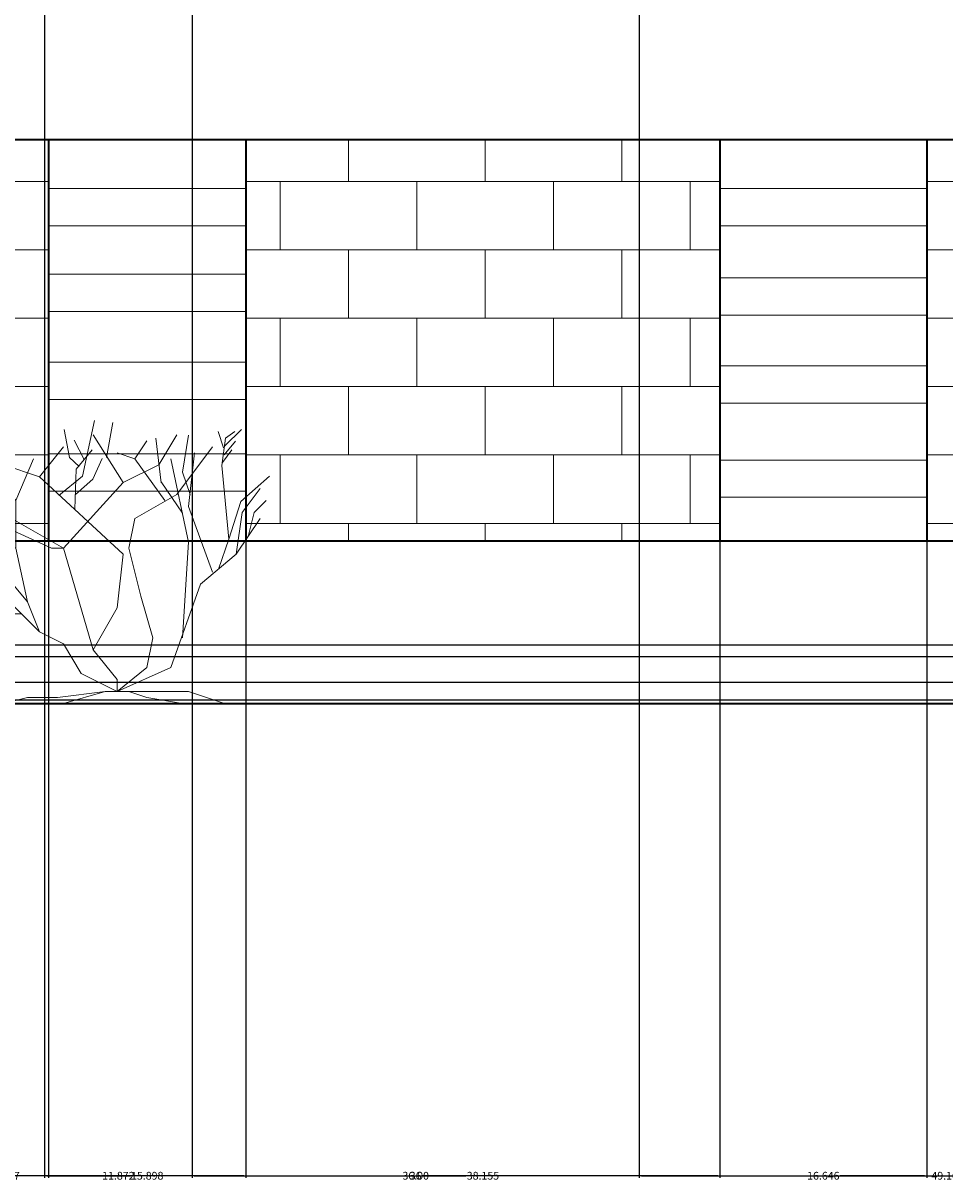
# Model space of a CAD drawing. Units: inches. Extents: x -13 to 809, y 112 to 656.
# Tile 7 of 55: x 111 to 186, y 112 to 205. Entities that reach past the tile are written whole.
import ezdxf

# ---------------------------------------------------------------- set-up
doc = ezdxf.new("R2010")
doc.units = ezdxf.units.IN
doc.header["$MEASUREMENT"] = 0
for name, color, linetype, lineweight in [('A-ANNO-DIMS', 2, 'Continuous', 18), ('A-ELEV', 7, 'Continuous', 35), ('A-ELEV-PATT', 8, 'Continuous', 13), ('L-PLNT', 3, 'Continuous', 18)]:
    doc.layers.add(name, color=color, linetype=linetype, lineweight=lineweight)
doc.styles.get("Standard").update_dxf_attribs({"font": 'arial.ttf'})
doc.dimstyles.get("Standard").update_dxf_attribs({"dimtxt": 0.625, "dimasz": 0.18, "dimexe": 0.18, "dimexo": 0.0625, "dimgap": 0.09, "dimtad": 0, "dimtih": 1, "dimtoh": 1, "dimdec": 4, "dimzin": 0, "dimdsep": 46, "dimlunit": 4, "dimtxsty": 'Standard', "dimcen": 0.09, "dimadec": 0, "dimazin": 0, "dimtfac": 1, "dimtdec": 4, "dimtofl": 0, "dimtmove": 0, "dimatfit": 3, "dimfxl": 1, "dimtolj": 1, "dimtzin": 0, "dimarcsym": 0})

# ---------------------------------------------------------------- blocks, each defined once
blk = doc.blocks.new('Shrub - elevation')
for p, q in [((-11.433, 18.289), (-10.457, 22.749)), ((-9.48, 19.775), (-8.992, 22.592)), ((-12.471, 19.775), (-12.898, 22.044)), ((-8.16, 17.76), (-10.56, 21.6)), ((-5.28, 19.2), (-3.84, 21.6)), ((-3.377, 18.602), (-2.888, 21.575)), ((-0.508, 21.888), (-0.081, 20.558)), ((0.041, 20.714), (1.384, 22.044)), ((0.102, 21.34), (0.835, 21.888)), ((-14.88, 18.24), (-12.96, 20.64)), ((-11.28, 19.619), (-12.104, 21.184)), ((-7.2, 19.68), (-6.24, 21.12)), ((-5.086, 17.741), (-5.513, 21.34)), ((-3.84, 16.8), (-0.96, 20.64)), ((-0.203, 19.149), (0.102, 21.34)), ((-0.02, 20.01), (0.896, 21.105)), ((-16.8, 16.32), (-15.36, 19.68)), ((-11.677, 19.071), (-12.471, 19.775)), ((-11.921, 18.836), (-10.64, 20.401)), ((-10.579, 18.054), (-9.846, 19.697)), ((-7.2, 19.68), (-8.64, 20.16)), ((-4.8, 16.32), (-7.2, 19.68)), ((-2.88, 12.96), (-4.32, 19.68)), ((-2.88, 15.84), (-2.4, 20.16)), ((-0.142, 19.384), (0.59, 20.401)), ((-16.8, 16.32), (-18.72, 18.72)), ((-14.88, 18.24), (-17.76, 19.2)), ((-12.043, 15.628), (-11.921, 18.836)), ((-8.16, 17.76), (-5.28, 19.2)), ((0.346, 13.203), (-0.203, 19.149)), ((-8.16, 12), (-14.88, 18.24)), ((-13.325, 16.724), (-11.433, 18.289)), ((-12.96, 12.48), (-8.16, 17.76)), ((-11.982, 16.802), (-10.579, 18.054)), ((-3.377, 15.315), (-5.086, 17.819)), ((-2.766, 16.802), (-3.377, 18.602)), ((1.323, 16.254), (3.642, 18.289)), ((-7.2, 14.88), (-3.84, 16.8)), ((1.44, 15.36), (2.88, 17.28)), ((-18.24, 11.04), (-21.755, 16.655)), ((-12.96, 12.48), (-19.68, 16.32)), ((-16.8, 12.48), (-16.8, 16.32)), ((-0.96, 10.56), (-2.88, 15.84)), ((0.346, 13.203), (1.323, 16.254)), ((2.4, 15.36), (3.36, 16.32)), ((0.96, 12), (1.44, 15.36)), ((1.92, 13.44), (2.4, 15.36)), ((-13.92, 12.48), (-19.2, 14.88)), ((-7.68, 12.48), (-7.2, 14.88)), ((0.96, 12), (2.88, 14.88)), ((-0.48, 10.8), (0.346, 13.203)), ((-16.8, 12.48), (-17.76, 12.96)), ((-15.84, 8.16), (-16.8, 12.48)), ((-12.96, 12.48), (-13.92, 12.48)), ((-10.56, 4.32), (-12.96, 12.48)), ((-6.72, 8.64), (-7.68, 12.48)), ((-3.36, 5.28), (-2.88, 12.96)), ((-17.76, 8.64), (-23.663, 11.961)), ((-18.24, 11.04), (-20.16, 11.52)), ((-8.64, 7.68), (-8.16, 12)), ((-1.92, 9.6), (0.96, 12)), ((-15.84, 8.16), (-18.24, 11.04)), ((-4.32, 2.88), (-1.92, 9.6)), ((-17.76, 8.64), (-23.128, 9.222)), ((-14.88, 5.76), (-17.76, 8.64)), ((-5.76, 5.28), (-6.72, 8.64)), ((-14.88, 5.76), (-15.84, 8.16)), ((-10.56, 4.32), (-8.64, 7.68)), ((-16.32, 7.2), (-18.24, 7.2)), ((-12.96, 4.8), (-14.88, 5.76)), ((-11.52, 2.4), (-12.96, 4.8)), ((-6.24, 2.88), (-5.76, 5.28)), ((-8.64, 1.92), (-10.56, 4.32)), ((-8.64, 0.96), (-4.32, 2.88)), ((-8.64, 0.96), (-6.24, 2.88)), ((-8.64, 0.96), (-11.52, 2.4)), ((-8.64, 0.96), (-8.64, 1.92)), ((-9.6, 0.96), (-13.44, 0.48)), ((-9.6, 0.96), (-12.96, 0)), ((-9.6, 0.96), (-7.68, 0.96)), ((-8.64, 0.96), (-2.88, 0.96)), ((-7.68, 0.96), (-6.24, 0.48)), ((-2.88, 0.96), (0, 0)), ((-15.84, 0.48), (-17.76, 0)), ((-13.44, 0.48), (-15.84, 0.48)), ((-6.24, 0.48), (-3.36, 0))]:
    blk.add_line(p, q)
blk = doc.blocks.new('*D12')
at = {"layer": 'A-ANNO-DIMS', "color": 0, "lineweight": -2, "transparency": 16777216}
for p, q in [((95.047, 306.457), (95.047, 112.34)), ((124.918, 210.457), (124.918, 112.34)), ((95.227, 112.52), (108.833, 112.52)), ((124.738, 112.52), (111.133, 112.52))]:
    blk.add_line(p, q, dxfattribs=at)
at = {"layer": 'A-ANNO-DIMS', "color": 0, "transparency": 16777216}
for points in [[(95.227, 112.55), (95.227, 112.49), (95.047, 112.52)], [(124.738, 112.55), (124.738, 112.49), (124.918, 112.52)]]:
    blk.add_solid(points, dxfattribs=at)
at = {"layer": 'Defpoints', "color": 0, "transparency": 16777216}
for p in [(95.047, 306.52), (124.918, 210.52), (124.918, 112.52)]:
    blk.add_point(p, dxfattribs=at)
at = {"layer": 'A-ANNO-DIMS', "color": 0, "transparency": 16777216, "insert": (109.983, 112.52), "char_height": 0.625, "attachment_point": 5}
blk.add_mtext('\\A1;29.87', dxfattribs=at)
blk = doc.blocks.new('*D13')
at = {"layer": 'A-ANNO-DIMS', "color": 0, "lineweight": -2, "transparency": 16777216}
for p, q in [((124.918, 210.457), (124.918, 112.34)), ((160.918, 210.457), (160.918, 112.34)), ((125.098, 112.52), (142.381, 112.52)), ((160.738, 112.52), (143.456, 112.52))]:
    blk.add_line(p, q, dxfattribs=at)
at = {"layer": 'A-ANNO-DIMS', "color": 0, "transparency": 16777216}
for points in [[(125.098, 112.55), (125.098, 112.49), (124.918, 112.52)], [(160.738, 112.55), (160.738, 112.49), (160.918, 112.52)]]:
    blk.add_solid(points, dxfattribs=at)
at = {"layer": 'Defpoints', "color": 0, "transparency": 16777216}
for p in [(124.918, 210.52), (160.918, 210.52), (160.918, 112.52)]:
    blk.add_point(p, dxfattribs=at)
at = {"layer": 'A-ANNO-DIMS', "color": 0, "transparency": 16777216, "insert": (142.918, 112.52), "char_height": 0.625, "attachment_point": 5}
blk.add_mtext('\\A1;36', dxfattribs=at)
blk = doc.blocks.new('*D14')
at = {"layer": 'A-ANNO-DIMS', "color": 0, "lineweight": -2, "transparency": 16777216}
for p, q in [((210.079, 223.038), (210.079, 112.34)), ((160.918, 210.457), (160.918, 112.34)), ((161.098, 112.52), (184.342, 112.52)), ((209.899, 112.52), (186.656, 112.52))]:
    blk.add_line(p, q, dxfattribs=at)
at = {"layer": 'A-ANNO-DIMS', "color": 0, "transparency": 16777216}
for points in [[(161.098, 112.55), (161.098, 112.49), (160.918, 112.52)], [(209.899, 112.55), (209.899, 112.49), (210.079, 112.52)]]:
    blk.add_solid(points, dxfattribs=at)
at = {"layer": 'Defpoints', "color": 0, "transparency": 16777216}
for p in [(210.079, 223.1), (160.918, 210.52), (210.079, 112.52)]:
    blk.add_point(p, dxfattribs=at)
at = {"layer": 'A-ANNO-DIMS', "color": 0, "transparency": 16777216, "insert": (185.499, 112.52), "char_height": 0.625, "attachment_point": 5}
blk.add_mtext('\\A1;49.16', dxfattribs=at)
blk = doc.blocks.new('*D85')
at = {"layer": 'A-ANNO-DIMS', "color": 0, "lineweight": -2, "transparency": 16777216}
for p, q in [((76.473, 195.828), (76.473, 112.34)), ((113.357, 195.828), (113.357, 112.34)), ((76.653, 112.52), (93.529, 112.52)), ((113.177, 112.52), (96.301, 112.52))]:
    blk.add_line(p, q, dxfattribs=at)
at = {"layer": 'A-ANNO-DIMS', "color": 0, "transparency": 16777216}
for points in [[(76.653, 112.55), (76.653, 112.49), (76.473, 112.52)], [(113.177, 112.55), (113.177, 112.49), (113.357, 112.52)]]:
    blk.add_solid(points, dxfattribs=at)
at = {"layer": 'Defpoints', "color": 0, "transparency": 16777216}
for p in [(76.473, 195.891), (113.357, 195.891), (113.357, 112.52)]:
    blk.add_point(p, dxfattribs=at)
at = {"layer": 'A-ANNO-DIMS', "color": 0, "transparency": 16777216, "insert": (94.915, 112.52), "char_height": 0.625, "attachment_point": 5}
blk.add_mtext('\\A1;36.884', dxfattribs=at)
blk = doc.blocks.new('*D86')
at = {"layer": 'A-ANNO-DIMS', "color": 0, "lineweight": -2, "transparency": 16777216}
for p, q in [((113.357, 195.828), (113.357, 112.34)), ((129.255, 195.828), (129.255, 112.34)), ((113.537, 112.52), (119.948, 112.52)), ((129.075, 112.52), (122.665, 112.52))]:
    blk.add_line(p, q, dxfattribs=at)
at = {"layer": 'A-ANNO-DIMS', "color": 0, "transparency": 16777216}
for points in [[(113.537, 112.55), (113.537, 112.49), (113.357, 112.52)], [(129.075, 112.55), (129.075, 112.49), (129.255, 112.52)]]:
    blk.add_solid(points, dxfattribs=at)
at = {"layer": 'Defpoints', "color": 0, "transparency": 16777216}
for p in [(113.357, 195.891), (129.255, 195.891), (129.255, 112.52)]:
    blk.add_point(p, dxfattribs=at)
at = {"layer": 'A-ANNO-DIMS', "color": 0, "transparency": 16777216, "insert": (121.306, 112.52), "char_height": 0.625, "attachment_point": 5}
blk.add_mtext('\\A1;15.898', dxfattribs=at)
blk = doc.blocks.new('*D87')
at = {"layer": 'A-ANNO-DIMS', "color": 0, "lineweight": -2, "transparency": 16777216}
for p, q in [((129.255, 195.828), (129.255, 112.34)), ((167.41, 195.828), (167.41, 112.34)), ((129.435, 112.52), (146.943, 112.52)), ((167.23, 112.52), (149.722, 112.52))]:
    blk.add_line(p, q, dxfattribs=at)
at = {"layer": 'A-ANNO-DIMS', "color": 0, "transparency": 16777216}
for points in [[(129.435, 112.55), (129.435, 112.49), (129.255, 112.52)], [(167.23, 112.55), (167.23, 112.49), (167.41, 112.52)]]:
    blk.add_solid(points, dxfattribs=at)
at = {"layer": 'Defpoints', "color": 0, "transparency": 16777216}
for p in [(129.255, 195.891), (167.41, 195.891), (167.41, 112.52)]:
    blk.add_point(p, dxfattribs=at)
at = {"layer": 'A-ANNO-DIMS', "color": 0, "transparency": 16777216, "insert": (148.332, 112.52), "char_height": 0.625, "attachment_point": 5}
blk.add_mtext('\\A1;38.155', dxfattribs=at)
blk = doc.blocks.new('*D88')
at = {"layer": 'A-ANNO-DIMS', "color": 0, "lineweight": -2, "transparency": 16777216}
for p, q in [((167.41, 195.828), (167.41, 112.34)), ((184.056, 195.828), (184.056, 112.34)), ((167.59, 112.52), (174.375, 112.52)), ((183.876, 112.52), (177.09, 112.52))]:
    blk.add_line(p, q, dxfattribs=at)
at = {"layer": 'A-ANNO-DIMS', "color": 0, "transparency": 16777216}
for points in [[(167.59, 112.55), (167.59, 112.49), (167.41, 112.52)], [(183.876, 112.55), (183.876, 112.49), (184.056, 112.52)]]:
    blk.add_solid(points, dxfattribs=at)
at = {"layer": 'Defpoints', "color": 0, "transparency": 16777216}
for p in [(167.41, 195.891), (184.056, 195.891), (184.056, 112.52)]:
    blk.add_point(p, dxfattribs=at)
at = {"layer": 'A-ANNO-DIMS', "color": 0, "transparency": 16777216, "insert": (175.733, 112.52), "char_height": 0.625, "attachment_point": 5}
blk.add_mtext('\\A1;16.646', dxfattribs=at)
blk = doc.blocks.new('*D89')
at = {"layer": 'A-ANNO-DIMS', "color": 0, "lineweight": -2, "transparency": 16777216}
for p, q in [((184.056, 195.828), (184.056, 112.34)), ((229.674, 195.828), (229.674, 112.34)), ((184.236, 112.52), (205.711, 112.52)), ((229.494, 112.52), (208.019, 112.52))]:
    blk.add_line(p, q, dxfattribs=at)
at = {"layer": 'A-ANNO-DIMS', "color": 0, "transparency": 16777216}
for points in [[(184.236, 112.55), (184.236, 112.49), (184.056, 112.52)], [(229.494, 112.55), (229.494, 112.49), (229.674, 112.52)]]:
    blk.add_solid(points, dxfattribs=at)
at = {"layer": 'Defpoints', "color": 0, "transparency": 16777216}
for p in [(184.056, 195.891), (229.674, 195.891), (229.674, 112.52)]:
    blk.add_point(p, dxfattribs=at)
at = {"layer": 'A-ANNO-DIMS', "color": 0, "transparency": 16777216, "insert": (206.865, 112.52), "char_height": 0.625, "attachment_point": 5}
blk.add_mtext('\\A1;45.62', dxfattribs=at)
blk = doc.blocks.new('*D107')
at = {"layer": 'A-ANNO-DIMS', "color": 0, "lineweight": -2, "transparency": 16777216}
for p, q in [((113.047, 324.457), (113.047, 112.34)), ((95.047, 306.457), (95.047, 112.34)), ((95.227, 112.52), (102.933, 112.52)), ((112.867, 112.52), (105.161, 112.52))]:
    blk.add_line(p, q, dxfattribs=at)
at = {"layer": 'A-ANNO-DIMS', "color": 0, "transparency": 16777216}
for points in [[(95.227, 112.55), (95.227, 112.49), (95.047, 112.52)], [(112.867, 112.55), (112.867, 112.49), (113.047, 112.52)]]:
    blk.add_solid(points, dxfattribs=at)
at = {"layer": 'Defpoints', "color": 0, "transparency": 16777216}
for p in [(113.047, 324.52), (95.047, 306.52), (113.047, 112.52)]:
    blk.add_point(p, dxfattribs=at)
at = {"layer": 'A-ANNO-DIMS', "color": 0, "transparency": 16777216, "insert": (104.047, 112.52), "char_height": 0.625, "attachment_point": 5}
blk.add_mtext('\\A1;18.00', dxfattribs=at)
blk = doc.blocks.new('*D109')
at = {"layer": 'A-ANNO-DIMS', "color": 0, "lineweight": -2, "transparency": 16777216}
for p, q in [((113.047, 324.457), (113.047, 112.34)), ((124.918, 324.457), (124.918, 112.34)), ((113.227, 112.52), (117.628, 112.52)), ((124.738, 112.52), (120.337, 112.52))]:
    blk.add_line(p, q, dxfattribs=at)
at = {"layer": 'A-ANNO-DIMS', "color": 0, "transparency": 16777216}
for points in [[(113.227, 112.55), (113.227, 112.49), (113.047, 112.52)], [(124.738, 112.55), (124.738, 112.49), (124.918, 112.52)]]:
    blk.add_solid(points, dxfattribs=at)
at = {"layer": 'Defpoints', "color": 0, "transparency": 16777216}
for p in [(113.047, 324.52), (124.918, 324.52), (124.918, 112.52)]:
    blk.add_point(p, dxfattribs=at)
at = {"layer": 'A-ANNO-DIMS', "color": 0, "transparency": 16777216, "insert": (118.983, 112.52), "char_height": 0.625, "attachment_point": 5}
blk.add_mtext('\\A1;11.872', dxfattribs=at)
blk = doc.blocks.new('*D110')
at = {"layer": 'A-ANNO-DIMS', "color": 0, "lineweight": -2, "transparency": 16777216}
for p, q in [((124.918, 324.457), (124.918, 112.34)), ((160.918, 324.457), (160.918, 112.34)), ((125.098, 112.52), (141.775, 112.52)), ((160.738, 112.52), (144.062, 112.52))]:
    blk.add_line(p, q, dxfattribs=at)
at = {"layer": 'A-ANNO-DIMS', "color": 0, "transparency": 16777216}
for points in [[(125.098, 112.55), (125.098, 112.49), (124.918, 112.52)], [(160.738, 112.55), (160.738, 112.49), (160.918, 112.52)]]:
    blk.add_solid(points, dxfattribs=at)
at = {"layer": 'Defpoints', "color": 0, "transparency": 16777216}
for p in [(124.918, 324.52), (160.918, 324.52), (160.918, 112.52)]:
    blk.add_point(p, dxfattribs=at)
at = {"layer": 'A-ANNO-DIMS', "color": 0, "transparency": 16777216, "insert": (142.918, 112.52), "char_height": 0.625, "attachment_point": 5}
blk.add_mtext('\\A1;36.00', dxfattribs=at)
blk = doc.blocks.new('*D111')
at = {"layer": 'A-ANNO-DIMS', "color": 0, "lineweight": -2, "transparency": 16777216}
for p, q in [((210.079, 361.229), (210.079, 112.34)), ((160.918, 324.457), (160.918, 112.34)), ((161.098, 112.52), (184.342, 112.52)), ((209.899, 112.52), (186.656, 112.52))]:
    blk.add_line(p, q, dxfattribs=at)
at = {"layer": 'A-ANNO-DIMS', "color": 0, "transparency": 16777216}
for points in [[(161.098, 112.55), (161.098, 112.49), (160.918, 112.52)], [(209.899, 112.55), (209.899, 112.49), (210.079, 112.52)]]:
    blk.add_solid(points, dxfattribs=at)
at = {"layer": 'Defpoints', "color": 0, "transparency": 16777216}
for p in [(210.079, 361.292), (160.918, 324.52), (210.079, 112.52)]:
    blk.add_point(p, dxfattribs=at)
at = {"layer": 'A-ANNO-DIMS', "color": 0, "transparency": 16777216, "insert": (185.499, 112.52), "char_height": 0.625, "attachment_point": 5}
blk.add_mtext('\\A1;49.16', dxfattribs=at)
blk = doc.blocks.new('*D115')
at = {"layer": 'A-ANNO-DIMS', "color": 0, "lineweight": -2, "transparency": 16777216}
for p, q in [((311.4, 210.785), (-12.099, 210.785)), ((-11.919, 210.605), (-11.919, 181.062)), ((-11.919, 150.7), (-11.919, 180.243)), ((311.637, 150.52), (-12.099, 150.52))]:
    blk.add_line(p, q, dxfattribs=at)
at = {"layer": 'A-ANNO-DIMS', "color": 0, "transparency": 16777216}
for points in [[(-11.949, 210.605), (-11.889, 210.605), (-11.919, 210.785)], [(-11.949, 150.7), (-11.889, 150.7), (-11.919, 150.52)]]:
    blk.add_solid(points, dxfattribs=at)
at = {"layer": 'Defpoints', "color": 0, "transparency": 16777216}
for p in [(-11.919, 210.785), (311.463, 210.785), (311.699, 150.52)]:
    blk.add_point(p, dxfattribs=at)
at = {"layer": 'A-ANNO-DIMS', "color": 0, "transparency": 16777216, "insert": (-11.919, 180.652), "char_height": 0.625, "attachment_point": 5}
blk.add_mtext('\\A1;60.27', dxfattribs=at)
blk = doc.blocks.new('*D117')
at = {"layer": 'A-ANNO-DIMS', "color": 0, "lineweight": -2, "transparency": 16777216}
for p, q in [((260.642, 154.272), (-12.099, 154.272)), ((-11.919, 154.092), (-11.919, 152.938)), ((-11.919, 150.965), (-11.919, 152.119)), ((258.04, 150.785), (-12.099, 150.785))]:
    blk.add_line(p, q, dxfattribs=at)
at = {"layer": 'A-ANNO-DIMS', "color": 0, "transparency": 16777216}
for points in [[(-11.949, 154.092), (-11.889, 154.092), (-11.919, 154.272)], [(-11.949, 150.965), (-11.889, 150.965), (-11.919, 150.785)]]:
    blk.add_solid(points, dxfattribs=at)
at = {"layer": 'Defpoints', "color": 0, "transparency": 16777216}
for p in [(260.705, 154.272), (-11.919, 150.785), (258.102, 150.785)]:
    blk.add_point(p, dxfattribs=at)
at = {"layer": 'A-ANNO-DIMS', "color": 0, "transparency": 16777216, "insert": (-11.919, 152.529), "char_height": 0.625, "attachment_point": 5}
blk.add_mtext('\\A1;3.487', dxfattribs=at)
blk = doc.blocks.new('*D131')
at = {"layer": 'A-ANNO-DIMS', "color": 0, "lineweight": -2, "transparency": 16777216}
for p, q in [((368.876, 155.214), (-12.099, 155.214)), ((-11.919, 155.034), (-11.919, 154.123)), ((-11.919, 152.394), (-11.919, 153.305)), ((365.876, 152.214), (-12.099, 152.214))]:
    blk.add_line(p, q, dxfattribs=at)
at = {"layer": 'A-ANNO-DIMS', "color": 0, "transparency": 16777216}
for points in [[(-11.949, 155.034), (-11.889, 155.034), (-11.919, 155.214)], [(-11.949, 152.394), (-11.889, 152.394), (-11.919, 152.214)]]:
    blk.add_solid(points, dxfattribs=at)
at = {"layer": 'Defpoints', "color": 0, "transparency": 16777216}
for p in [(368.938, 155.214), (-11.919, 152.214), (365.938, 152.214)]:
    blk.add_point(p, dxfattribs=at)
at = {"layer": 'A-ANNO-DIMS', "color": 0, "transparency": 16777216, "insert": (-11.919, 153.714), "char_height": 0.625, "attachment_point": 5}
blk.add_mtext('\\A1;3.00', dxfattribs=at)

msp = doc.modelspace()

# ---------------------------------------------------------------- hatches: boundary and pattern name
at = {"layer": 'A-ELEV-PATT'}
h = msp.add_hatch(dxfattribs=at)
h.set_pattern_fill('BRICK', color=256, scale=22)
h.paths.add_polyline_path([(113.3574, 195.8907), (76.4733, 195.8907), (76.4733, 163.5637), (113.3574, 163.5637)])
h.paths.add_polyline_path([(167.4098, 195.8907), (129.2551, 195.8907), (129.2551, 163.5637), (167.4098, 163.5637)])
h.paths.add_polyline_path([(229.6736, 195.8907), (184.0557, 195.8907), (184.0557, 163.5637), (229.6736, 163.5637)])

# ---------------------------------------------------------------- linework, layer by layer
at = {"layer": 'A-ELEV'}
for p, q in [((113.3574, 195.8907), (113.3574, 163.5637)), ((129.2551, 195.8907), (129.2551, 163.5637)), ((167.4098, 195.8907), (167.4098, 163.5637)), ((184.0557, 195.8907), (184.0557, 163.5637)), ((109.5888, 150.5199), (649.5888, 150.5199))]:
    msp.add_line(p, q, dxfattribs=at)
msp.add_lwpolyline([(76.4733, 195.8907), (229.6736, 195.8907), (229.6736, 163.5637), (76.4733, 163.5637)], close=True, dxfattribs=at)
at = {"layer": 'A-ELEV-PATT'}
for p, q in [((113.3574, 191.9338), (129.2551, 191.9338)), ((167.4098, 191.9338), (184.0557, 191.9338)), ((113.3574, 188.9338), (129.2551, 188.9338)), ((167.4098, 188.9338), (184.0557, 188.9338)), ((113.3574, 185.0499), (129.2551, 185.0499)), ((167.4098, 184.7549), (184.0557, 184.7549)), ((113.3574, 182.0499), (129.2551, 182.0499)), ((167.4098, 181.7549), (184.0557, 181.7549)), ((113.3574, 177.9693), (129.2551, 177.9693)), ((167.4098, 177.6743), (184.0557, 177.6743)), ((113.3574, 174.9693), (129.2551, 174.9693)), ((167.4098, 174.6743), (184.0557, 174.6743)), ((113.3574, 170.5937), (129.2551, 170.5937)), ((167.4098, 170.102), (184.0557, 170.102)), ((113.3574, 167.5937), (129.2551, 167.5937)), ((167.4098, 167.102), (184.0557, 167.102))]:
    msp.add_line(p, q, dxfattribs=at)

# ---------------------------------------------------------------- block references
at = {"layer": 'L-PLNT'}
msp.add_blockref('Shrub - elevation', (127.517, 150.5199), dxfattribs=at)

# ---------------------------------------------------------------- dimensions: what is measured, and where the dimension line sits
at = {"layer": 'A-ANNO-DIMS'}
for base, p1, p2, override, picture, middle in [((210.0791, 112.5199), (160.9184, 324.5199), (210.0791, 361.2915), {"dimdec": 2, "dimlfac": 1, "dimrnd": 0, "dimzin": 0, "dimdsep": 46, "dimlunit": 2}, '*D111', (185.4988, 112.5199)), ((113.0469, 112.5199), (95.0469, 306.5199), (113.0469, 324.5199), {"dimdec": 2, "dimlfac": 1, "dimrnd": 0, "dimzin": 0, "dimdsep": 46, "dimlunit": 2}, '*D107', (104.0469, 112.5199)), ((124.91845, 112.51989), (113.04686, 324.51989), (124.91845, 324.51989), {"dimdec": 3, "dimlfac": 1, "dimrnd": 0, "dimzin": 0, "dimdsep": 46, "dimlunit": 2}, '*D109', (118.98265, 112.51989)), ((160.9184, 112.5199), (124.9184, 324.5199), (160.9184, 324.5199), {"dimdec": 2, "dimlfac": 1, "dimrnd": 0, "dimzin": 0, "dimdsep": 46, "dimlunit": 2}, '*D110', (142.9184, 112.5199)), ((124.9184, 112.5199), (95.0469, 306.5199), (124.9184, 210.5199), {"dimdec": 2, "dimlfac": 1, "dimrnd": 0, "dimzin": 0, "dimdsep": 46, "dimlunit": 2}, '*D12', (109.9827, 112.5199)), ((210.0791, 112.5199), (160.9184, 210.5199), (210.0791, 223.1), {"dimdec": 2, "dimlfac": 1, "dimrnd": 0, "dimzin": 0, "dimdsep": 46, "dimlunit": 2}, '*D14', (185.4988, 112.5199)), ((160.9184, 112.5199), (124.9184, 210.5199), (160.9184, 210.5199), {"dimdec": 0, "dimlfac": 1, "dimrnd": 0, "dimzin": 0, "dimdsep": 46, "dimlunit": 2}, '*D13', (142.9184, 112.5199)), ((113.3574, 112.5199), (76.4733, 195.8907), (113.3574, 195.8907), {"dimdec": 3, "dimlfac": 1, "dimrnd": 0, "dimzin": 0, "dimdsep": 46, "dimlunit": 2}, '*D85', (94.9153, 112.5199)), ((129.2551, 112.5199), (113.3574, 195.8907), (129.2551, 195.8907), {"dimdec": 3, "dimlfac": 1, "dimrnd": 0, "dimzin": 0, "dimdsep": 46, "dimlunit": 2}, '*D86', (121.3063, 112.5199)), ((167.4098, 112.5199), (129.2551, 195.8907), (167.4098, 195.8907), {"dimdec": 3, "dimlfac": 1, "dimrnd": 0, "dimzin": 0, "dimdsep": 46, "dimlunit": 2}, '*D87', (148.3325, 112.5199)), ((184.0557, 112.5199), (167.4098, 195.8907), (184.0557, 195.8907), {"dimdec": 3, "dimlfac": 1, "dimrnd": 0, "dimzin": 0, "dimdsep": 46, "dimlunit": 2}, '*D88', (175.7327, 112.5199)), ((229.6736, 112.5199), (184.0557, 195.8907), (229.6736, 195.8907), {"dimdec": 2, "dimlfac": 1, "dimrnd": 0, "dimzin": 0, "dimdsep": 46, "dimlunit": 2}, '*D89', (206.8646, 112.5199))]:
    dim = msp.add_linear_dim(base=base, p1=p1, p2=p2, dimstyle='Standard', override=override, dxfattribs=at)
    dim.commit()
    dim.dimension.update_dxf_attribs({"geometry": picture, "text_midpoint": middle})
for base, p1, p2, override, picture, middle in [((-11.91915, 210.78493), (311.6991, 150.51989), (311.46269, 210.78493), {"dimdec": 2, "dimlfac": 1, "dimrnd": 0, "dimzin": 0, "dimdsep": 46, "dimlunit": 2}, '*D115', (-11.91915, 180.65241)), ((-11.9191, 152.2141), (368.9383, 155.2141), (365.9383, 152.2141), {"dimdec": 2, "dimlfac": 1, "dimrnd": 0, "dimzin": 0, "dimdsep": 46, "dimlunit": 2}, '*D131', (-11.9191, 153.7141)), ((-11.9191, 150.7849), (260.7048, 154.2723), (258.1022, 150.7849), {"dimdec": 3, "dimlfac": 1, "dimrnd": 0, "dimzin": 0, "dimdsep": 46, "dimlunit": 2}, '*D117', (-11.9191, 152.5286))]:
    dim = msp.add_linear_dim(base=base, p1=p1, p2=p2, angle=90, dimstyle='Standard', override=override, dxfattribs=at)
    dim.commit()
    dim.dimension.update_dxf_attribs({"geometry": picture, "text_midpoint": middle})

doc.saveas('drawing.dxf')
